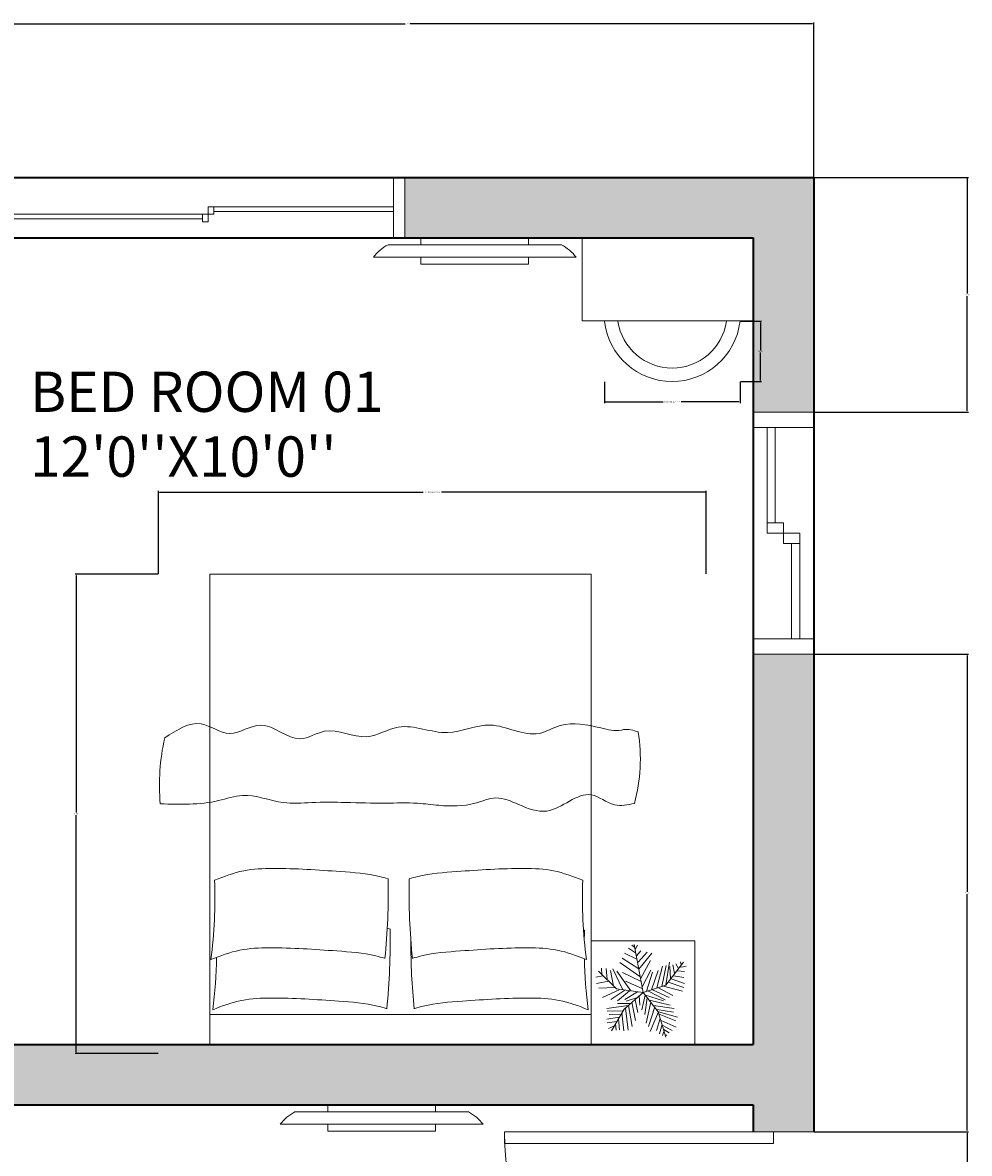
# Model space of a CAD drawing. Units: inches. Extents: x 1789 to 2841, y 3180 to 3702.
# Tile 7 of 14: x 2208 to 2348, y 3510 to 3678. Entities that reach past the tile are written whole.
import ezdxf

# ---------------------------------------------------------------- set-up
doc = ezdxf.new("R2010")
doc.units = ezdxf.units.IN
doc.header["$MEASUREMENT"] = 0
for name, color, linetype, lineweight in [('A-ANNO-DIMS', 2, 'Continuous', 18), ('A-AREA-IDEN', 7, 'Continuous', 18), ('A-EQPM', 8, 'Continuous', 18), ('A-WALL', 40, 'Continuous', 35), ('A-WALL-PATT', 252, 'Continuous', 13), ('DORS', 70, 'Continuous', 18), ('FURNITURE', 34, 'Continuous', 18), ('WINDOWS', 130, 'Continuous', 18)]:
    doc.layers.add(name, color=color, linetype=linetype, lineweight=lineweight)
doc.styles.get("Standard").update_dxf_attribs({"font": 'arial.ttf'})
doc.dimstyles.get("Standard").update_dxf_attribs({"dimtxt": 0.18, "dimasz": 0.18, "dimexe": 0.18, "dimexo": 0.0625, "dimgap": 0.09, "dimtad": 0, "dimtih": 1, "dimtoh": 1, "dimdec": 0, "dimzin": 0, "dimdsep": 46, "dimlunit": 3, "dimtxsty": 'Standard', "dimcen": 0.09, "dimadec": 0, "dimazin": 0, "dimtfac": 1, "dimtdec": 0, "dimtofl": 0, "dimtmove": 0, "dimatfit": 3, "dimfxl": 1, "dimtolj": 1, "dimtzin": 0, "dimarcsym": 0})

# ---------------------------------------------------------------- blocks, each defined once
blk = doc.blocks.new('HYJ')
for p, q in [((2236.02, 3650.77), (2262.74, 3650.77)), ((2206.12, 3649.67), (2234.3, 3649.67)), ((2206.12, 3649), (2234.3, 3649)), ((2236.02, 3650.11), (2262.74, 3650.11))]:
    blk.add_line(p, q)
for points in [[(2204.43, 3646.16), (2264.43, 3646.16), (2264.43, 3655.16), (2204.43, 3655.16)], [(2204.43, 3655.16), (2206.12, 3655.16), (2206.12, 3646.16), (2204.43, 3646.16)], [(2264.43, 3655.16), (2262.74, 3655.16), (2262.74, 3646.16), (2264.43, 3646.16)], [(2235.16, 3650.77), (2236.02, 3650.77), (2236.02, 3649.67), (2235.16, 3649.67)], [(2234.3, 3649.67), (2235.16, 3649.67), (2235.16, 3648.56), (2234.3, 3648.56)]]:
    blk.add_lwpolyline(points, close=True)
blk = doc.blocks.new('KIK')
for p, q in [((2336.3, 3607.04), (2336.3, 3621.23)), ((2337.52, 3607.04), (2337.52, 3621.23)), ((2339.95, 3603.98), (2339.95, 3589.79)), ((2341.17, 3603.98), (2341.17, 3589.79))]:
    blk.add_line(p, q)
for points in [[(2343.23, 3623.51), (2343.23, 3587.51), (2334.23, 3587.51), (2334.23, 3623.51)], [(2343.23, 3623.51), (2334.23, 3623.51), (2334.23, 3621.23), (2343.23, 3621.23)], [(2338.73, 3605.51), (2336.3, 3605.51), (2336.3, 3607.04), (2338.73, 3607.04)], [(2341.17, 3603.98), (2338.73, 3603.98), (2338.73, 3605.51), (2341.17, 3605.51)], [(2343.23, 3587.51), (2334.23, 3587.51), (2334.23, 3589.79), (2343.23, 3589.79)]]:
    blk.add_lwpolyline(points, close=True)
blk = doc.blocks.new('GTGTG')
for points in [[(2266.82, 3646.16), (2282.82, 3646.16), (2282.82, 3645.14), (2266.82, 3645.14)], [(2266.82, 3643.29), (2282.82, 3643.29), (2282.82, 3642.27), (2266.82, 3642.27)]]:
    blk.add_lwpolyline(points, close=True)
for points in [[(2261.92, 3645.14), (2287.72, 3645.14)], [(2289.9, 3643.29), (2259.74, 3643.29)]]:
    blk.add_lwpolyline(points)
for centre, start, end in [((2265.21, 3639.05), 118.4184, 142.2436), ((2284.43, 3639.05), 37.7564, 61.5816)]:
    blk.add_arc(centre, 6.92, start, end)
blk = doc.blocks.new('*U26')
for p, q in [((0, 0), (0, -6)), ((40, 0), (40, -6))]:
    blk.add_line(p, q)
blk.add_lwpolyline([(0, 0), (0, 40), (1.75, 40), (1.75, 0)], close=True)
blk.add_arc((0, 0), 40, 0, 90)
blk = doc.blocks.new('*U22')
for p, q in [((-10.186, 53.64), (-13.084, 55.962)), ((0, 0), (-10.5, 57)), ((-9.099, 51.782), (-6.563, 55.962)), ((-5.114, 28.097), (-24.676, 40.636)), ((-7.288, 39.707), (-21.778, 46.673)), ((-8.737, 47.138), (-17.069, 52.711)), ((-7.65, 43.423), (-2.578, 49.46)), ((-5.839, 35.992), (4.667, 48.067)), ((-5.114, 27.632), (10.463, 46.673)), ((-48.585, 21.131), (-49.309, 29.026)), ((-43.513, 28.561), (-42.427, 15.558)), ((-35.544, 28.097), (-24.314, 3.947)), ((-3.665, 19.273), (-27.574, 35.527)), ((-2.941, 16.486), (8.652, 37.85)), ((16.259, 5.805), (23.142, 31.348)), ((22.055, 7.198), (27.489, 32.277)), ((27, 9), (48, 36)), ((27.127, 9.056), (31.112, 35.992)), ((31.836, 30.883), (32.561, 16.486)), ((35.096, 32.741), (37.27, 22.524)), ((38.719, 34.134), (41.979, 28.561)), ((43.791, 29.954), (51.036, 30.883)), ((44.153, 36.456), (45.239, 32.741)), ((-47.498, 19.737), (-55.83, 18.344)), ((-40.615, 13.7), (-55.105, 10.913)), ((-31.5, 4.5), (-52.5, 25.5)), ((-38.442, 26.239), (-34.819, 7.663)), ((-14.533, 2.09), (-30.834, 25.31)), ((-24.314, 23.917), (-2.941, 13.7)), ((-20.691, 13.7), (-1.129, 4.876)), ((-1.129, 6.734), (9.014, 26.704)), ((3.942, 1.625), (11.187, 24.381)), ((10.101, 3.483), (17.708, 26.239)), ((33.285, 16.486), (48.862, 10.913)), ((36.183, 19.737), (48.137, 17.88)), ((40.53, 25.775), (48.862, 24.846)), ((-33.37, 6.269), (-52.207, 5.34)), ((-28.299, 3.483), (-47.86, -5.805)), ((-21.416, 3.018), (-38.079, -8.128)), ((0, 0), (-31.5, 4.5)), ((-15.982, 2.09), (-30.11, -9.521)), ((0, 0), (-22.5, -19.5)), ((-6.563, 1.161), (-21.416, -8.128)), ((0, 0), (27, 9)), ((0, 0), (18, -22.5)), ((6.478, 1.625), (26.04, -8.592)), ((11.187, 3.483), (30.749, -5.805)), ((18.07, 5.805), (35.096, -3.483)), ((24.229, 7.663), (46.688, 1.625)), ((29.662, 12.307), (48.137, 6.269)), ((-15.257, -12.772), (-30.11, -12.772)), ((-6.563, -5.805), (-19.967, -9.985)), ((-13.446, -11.378), (-8.737, -32.741)), ((-9.461, -8.592), (-6.201, -23.453)), ((-4.752, -3.483), (-3.665, -14.629)), ((2.493, -3.019), (-1.491, -20.202)), ((1.769, -2.555), (24.229, -9.521)), ((5.029, -6.27), (2.131, -25.775)), ((9.014, -11.378), (3.58, -35.992)), ((7.565, -9.056), (32.198, -14.629)), ((-17.431, -15.094), (-42.789, -18.809)), ((-24.314, -21.596), (-42.427, -22.06)), ((-26.849, -26.24), (-40.253, -25.775)), ((-22.5, -19.5), (-37.5, -45)), ((-25.038, -23.918), (-22.865, -45.281)), ((-20.691, -18.345), (-17.793, -44.352)), ((-17.069, -15.094), (-12.721, -40.172)), ((14.085, -16.951), (6.478, -40.172)), ((18.07, -22.524), (8.289, -45.745)), ((12.274, -15.094), (36.907, -18.809)), ((16.259, -19.738), (36.183, -22.989)), ((18, -22.5), (27, -52.5)), ((18.433, -22.524), (40.53, -29.026)), ((19.157, -25.311), (38.719, -33.206)), ((-28.299, -29.026), (-42.789, -31.348)), ((-30.834, -34.135), (-42.427, -35.528)), ((-34.457, -39.708), (-40.978, -42.494)), ((-32.646, -36.921), (-31.921, -44.352)), ((-29.023, -30.884), (-27.936, -43.887)), ((20.244, -30.419), (15.897, -44.816)), ((22.78, -37.85), (19.519, -48.532)), ((21.331, -32.741), (39.081, -40.636)), ((22.78, -38.314), (34.372, -44.816)), ((24.591, -45.745), (23.142, -50.854)), ((24.591, -43.423), (30.749, -47.603)), ((26.764, -49.925), (28.213, -50.854))]:
    blk.add_line(p, q)
blk = doc.blocks.new('BEDD')
for points in [[(2235.4, 3526.16), (2292.14, 3526.16), (2292.14, 3596.12), (2235.4, 3596.12)], [(2292.14, 3526.16), (2307.57, 3526.16), (2307.57, 3541.59), (2292.14, 3541.59)], [(2235.4, 3526.16), (2292.14, 3526.16), (2292.14, 3530.61), (2235.4, 3530.61)]]:
    blk.add_lwpolyline(points, close=True)
for centre, radius, start, end in [((2259.99, 3564.78), 32.07, 167.4063, 185.0216), ((2273.81, 3568.71), 25.64, 344.9042, 8.8372), ((2163.47, 3548.06), 72.69, 352.674, 2.0029), ((2165.57, 3548.81), 96.38, 354.1175, 1.1854), ((2361.42, 3548.81), 96.38, 178.8146, 185.8825), ((2363.52, 3548.06), 72.69, 177.9971, 187.326), ((2165.85, 3541.35), 96.38, 354.1175, 1.1854), ((2363.79, 3540.6), 72.69, 177.9971, 179.1531), ((2361.69, 3541.35), 96.38, 179.877, 185.8825), ((2163.75, 3540.6), 72.69, 352.674, 358.8312), ((2363.79, 3540.6), 72.69, 181.3344, 187.326)]:
    blk.add_arc(centre, radius, start, end)
for points, knots in [([(2228.7, 3571.77), (2230.5, 3572.97), (2233.69, 3575.11), (2238.44, 3571.24), (2243.48, 3575.3), (2248.08, 3570.3), (2253.24, 3573.93), (2258.37, 3570.76), (2264.15, 3574.63), (2270.52, 3571.37), (2277.36, 3575.01), (2283.2, 3571.25), (2288.29, 3574.45), (2292.59, 3573.51), (2295.73, 3572.7), (2297.56, 3573.17), (2298.4, 3572.89), (2299.15, 3572.65)], [0, 0, 0, 0, 5.813057, 10.291797, 15.071674, 21.264477, 25.062958, 31.395117, 36.284741, 43.6566, 50.0956, 57.47363, 60.824937, 66.871309, 69.965772, 70.260383, 72.512122, 72.512122, 72.512122, 72.512122]), ([(2228.05, 3561.97), (2230.96, 3561.87), (2235.09, 3561.73), (2241.08, 3563.86), (2245.67, 3561.8), (2250.85, 3562.25), (2255.91, 3562.17), (2261.15, 3562), (2265.78, 3562.19), (2270.21, 3561.59), (2274.18, 3561.57), (2278.08, 3563.31), (2281.58, 3561.74), (2286.46, 3559.73), (2291.21, 3564.99), (2295.28, 3561.31), (2297.57, 3561.81), (2298.57, 3562.03)], [0, 0, 0, 0, 8.669632, 12.310458, 18.461416, 22.693385, 27.790985, 33.658819, 38.43562, 41.630677, 47.052462, 50.224855, 53.725722, 58.058029, 65.069701, 68.862462, 71.815525, 71.815525, 71.815525, 71.815525]), ([(2236.12, 3550.6), (2237.54, 3551.15), (2240.34, 3552.23), (2246.72, 3552.46), (2253.43, 3551.99), (2259.2, 3551.57), (2261.51, 3550.92), (2261.93, 3550.8)], [0, 0, 0, 0, 4.544245, 8.926813, 18.957656, 24.819591, 26.148375, 26.148375, 26.148375, 26.148375]), ([(2290.87, 3550.6), (2289.45, 3551.15), (2286.65, 3552.23), (2280.27, 3552.46), (2273.56, 3551.99), (2267.8, 3551.57), (2265.49, 3550.92), (2265.06, 3550.8)], [0, 0, 0, 0, 4.544245, 8.926813, 18.957656, 24.819591, 26.148375, 26.148375, 26.148375, 26.148375]), ([(2235.57, 3538.79), (2236.99, 3539.34), (2239.79, 3540.42), (2246.18, 3540.65), (2252.88, 3540.18), (2258.65, 3539.76), (2260.96, 3539.11), (2261.38, 3538.99)], [0, 0, 0, 0, 4.544245, 8.926813, 18.957656, 24.819591, 26.148375, 26.148375, 26.148375, 26.148375]), ([(2291.42, 3538.79), (2290, 3539.34), (2287.2, 3540.42), (2280.82, 3540.65), (2274.11, 3540.18), (2268.34, 3539.76), (2266.03, 3539.11), (2265.61, 3538.99)], [0, 0, 0, 0, 4.544245, 8.926813, 18.957656, 24.819591, 26.148375, 26.148375, 26.148375, 26.148375]), ([(2235.84, 3531.33), (2237.27, 3531.88), (2240.06, 3532.96), (2246.45, 3533.19), (2253.15, 3532.71), (2258.92, 3532.3), (2261.23, 3531.65), (2261.66, 3531.53)], [0, 0, 0, 0, 4.544245, 8.926813, 18.957656, 24.819591, 26.148375, 26.148375, 26.148375, 26.148375]), ([(2291.69, 3531.33), (2290.27, 3531.88), (2287.47, 3532.96), (2281.09, 3533.19), (2274.39, 3532.71), (2268.62, 3532.3), (2266.31, 3531.65), (2265.88, 3531.53)], [0, 0, 0, 0, 4.544245, 8.926813, 18.957656, 24.819591, 26.148375, 26.148375, 26.148375, 26.148375])]:
    blk.add_open_spline(points, degree=3, knots=knots)
for points in [[(2261.81, 3543.46), (2261.94, 3543.42), (2262.07, 3543.38), (2262.21, 3543.34)], [(2291.15, 3543.14), (2291.09, 3543.16), (2291.04, 3543.18), (2290.99, 3543.2)]]:
    blk.add_open_spline(points, degree=3)
at = {"xscale": 0.1258179792922857, "yscale": 0.1258179792922857, "zscale": 0.1258179792922857}
blk.add_blockref('*U22', (2299.85, 3533.87), dxfattribs=at)
blk = doc.blocks.new('CHAIR-DESK-ROUND')
for radius, start, end in [(10.16, 186.7458, 353.2542), (8.16, 188.4094, 351.5906)]:
    blk.add_arc((10.09, 10.16), radius, start, end)
blk = doc.blocks.new('*D55')
at = {"layer": 'A-ANNO-DIMS', "color": 0, "lineweight": -2, "transparency": 16777216}
for p, q in [((2227.76, 3596.18), (2227.76, 3608.52)), ((2227.94, 3608.34), (2267.14, 3608.34)), ((2309.08, 3608.34), (2269.88, 3608.34)), ((2309.26, 3596.18), (2309.26, 3608.52))]:
    blk.add_line(p, q, dxfattribs=at)
at = {"layer": 'A-ANNO-DIMS', "color": 0, "transparency": 16777216}
for points in [[(2227.94, 3608.37), (2227.94, 3608.31), (2227.76, 3608.34)], [(2309.08, 3608.37), (2309.08, 3608.31), (2309.26, 3608.34)]]:
    blk.add_solid(points, dxfattribs=at)
at = {"layer": 'Defpoints', "color": 0, "transparency": 16777216}
for p in [(2309.26, 3608.34), (2227.76, 3596.12), (2309.26, 3596.12)]:
    blk.add_point(p, dxfattribs=at)
at = {"layer": 'A-ANNO-DIMS', "color": 0, "transparency": 16777216, "insert": (2268.51, 3608.34), "char_height": 0.18, "attachment_point": 5}
blk.add_mtext('\\A1;DOUBLE BED 81 TYP.', dxfattribs=at)
blk = doc.blocks.new('*D56')
at = {"layer": 'A-ANNO-DIMS', "color": 0, "lineweight": -2, "transparency": 16777216}
for p, q in [((2227.7, 3596.12), (2215.36, 3596.12)), ((2215.54, 3595.94), (2215.54, 3560.65)), ((2215.54, 3525.01), (2215.54, 3560.29)), ((2227.7, 3524.83), (2215.36, 3524.83))]:
    blk.add_line(p, q, dxfattribs=at)
at = {"layer": 'A-ANNO-DIMS', "color": 0, "transparency": 16777216}
for points in [[(2215.51, 3595.94), (2215.57, 3595.94), (2215.54, 3596.12)], [(2215.51, 3525.01), (2215.57, 3525.01), (2215.54, 3524.83)]]:
    blk.add_solid(points, dxfattribs=at)
at = {"layer": 'Defpoints', "color": 0, "transparency": 16777216}
for p in [(2215.54, 3596.12), (2227.76, 3596.12), (2227.76, 3524.83)]:
    blk.add_point(p, dxfattribs=at)
at = {"layer": 'A-ANNO-DIMS', "color": 0, "transparency": 16777216, "insert": (2215.54, 3560.47), "char_height": 0.18, "attachment_point": 5}
blk.add_mtext('\\A1;71 TYP.', dxfattribs=at)
blk = doc.blocks.new('*D75')
at = {"layer": 'A-ANNO-DIMS', "color": 0, "lineweight": -2, "transparency": 16777216}
for p, q in [((2294.1, 3624.73), (2294.1, 3621.58)), ((2314.28, 3624.73), (2314.28, 3621.58)), ((2294.28, 3621.76), (2302.86, 3621.76)), ((2314.1, 3621.76), (2305.52, 3621.76))]:
    blk.add_line(p, q, dxfattribs=at)
at = {"layer": 'A-ANNO-DIMS', "color": 0, "transparency": 16777216}
for points in [[(2294.28, 3621.79), (2294.28, 3621.73), (2294.1, 3621.76)], [(2314.1, 3621.79), (2314.1, 3621.73), (2314.28, 3621.76)]]:
    blk.add_solid(points, dxfattribs=at)
at = {"layer": 'Defpoints', "color": 0, "transparency": 16777216}
for p in [(2294.1, 3624.79), (2314.28, 3624.79), (2314.28, 3621.76)]:
    blk.add_point(p, dxfattribs=at)
at = {"layer": 'A-ANNO-DIMS', "color": 0, "transparency": 16777216, "insert": (2304.19, 3621.76), "char_height": 0.18, "attachment_point": 5}
blk.add_mtext('\\A1;DESK CHAIR 20 TYP.', dxfattribs=at)
blk = doc.blocks.new('*D76')
at = {"layer": 'A-ANNO-DIMS', "color": 0, "lineweight": -2, "transparency": 16777216}
for p, q in [((2314.34, 3633.76), (2317.49, 3633.76)), ((2317.31, 3633.58), (2317.31, 3629.46)), ((2317.31, 3624.97), (2317.31, 3629.09)), ((2314.34, 3624.79), (2317.49, 3624.79))]:
    blk.add_line(p, q, dxfattribs=at)
at = {"layer": 'A-ANNO-DIMS', "color": 0, "transparency": 16777216}
for points in [[(2317.28, 3633.58), (2317.34, 3633.58), (2317.31, 3633.76)], [(2317.28, 3624.97), (2317.34, 3624.97), (2317.31, 3624.79)]]:
    blk.add_solid(points, dxfattribs=at)
at = {"layer": 'Defpoints', "color": 0, "transparency": 16777216}
for p in [(2314.28, 3633.76), (2317.31, 3633.76), (2314.28, 3624.79)]:
    blk.add_point(p, dxfattribs=at)
at = {"layer": 'A-ANNO-DIMS', "color": 0, "transparency": 16777216, "insert": (2317.31, 3629.28), "char_height": 0.18, "attachment_point": 5}
blk.add_mtext('\\A1;9 TYP.', dxfattribs=at)
blk = doc.blocks.new('*D85')
at = {"layer": 'A-ANNO-DIMS', "color": 0, "lineweight": -2, "transparency": 16777216}
for p, q in [((2204.43, 3655.22), (2204.43, 3678.19)), ((2204.61, 3678.01), (2264.45, 3678.01)), ((2325.05, 3678.01), (2265.22, 3678.01)), ((2325.23, 3655.22), (2325.23, 3678.19))]:
    blk.add_line(p, q, dxfattribs=at)
at = {"layer": 'A-ANNO-DIMS', "color": 0, "transparency": 16777216}
for points in [[(2204.61, 3678.04), (2204.61, 3677.98), (2204.43, 3678.01)], [(2325.05, 3678.04), (2325.05, 3677.98), (2325.23, 3678.01)]]:
    blk.add_solid(points, dxfattribs=at)
at = {"layer": 'Defpoints', "color": 0, "transparency": 16777216}
for p in [(2325.23, 3678.01), (2204.43, 3655.16), (2325.23, 3655.16)]:
    blk.add_point(p, dxfattribs=at)
at = {"layer": 'A-ANNO-DIMS', "color": 0, "transparency": 16777216, "insert": (2264.83, 3678.01), "char_height": 0.18, "attachment_point": 5}
blk.add_mtext('\\A1;120.8', dxfattribs=at)
blk = doc.blocks.new('*D86')
at = {"layer": 'A-ANNO-DIMS', "color": 0, "lineweight": -2, "transparency": 16777216}
for p, q in [((2325.3, 3655.16), (2348.26, 3655.16)), ((2348.08, 3654.98), (2348.08, 3637.88)), ((2348.08, 3620.41), (2348.08, 3637.51)), ((2325.3, 3620.23), (2348.26, 3620.23))]:
    blk.add_line(p, q, dxfattribs=at)
at = {"layer": 'A-ANNO-DIMS', "color": 0, "transparency": 16777216}
for points in [[(2348.05, 3654.98), (2348.11, 3654.98), (2348.08, 3655.16)], [(2348.05, 3620.41), (2348.11, 3620.41), (2348.08, 3620.23)]]:
    blk.add_solid(points, dxfattribs=at)
at = {"layer": 'Defpoints', "color": 0, "transparency": 16777216}
for p in [(2325.23, 3655.16), (2325.23, 3620.23), (2348.08, 3620.23)]:
    blk.add_point(p, dxfattribs=at)
at = {"layer": 'A-ANNO-DIMS', "color": 0, "transparency": 16777216, "insert": (2348.08, 3637.69), "char_height": 0.18, "attachment_point": 5}
blk.add_mtext('\\A1;34.93', dxfattribs=at)
blk = doc.blocks.new('*D87')
at = {"layer": 'A-ANNO-DIMS', "color": 0, "lineweight": -2, "transparency": 16777216}
for p, q in [((2325.3, 3584.23), (2348.26, 3584.23)), ((2348.08, 3584.05), (2348.08, 3548.88)), ((2348.08, 3513.34), (2348.08, 3548.51)), ((2325.3, 3513.16), (2348.26, 3513.16))]:
    blk.add_line(p, q, dxfattribs=at)
at = {"layer": 'A-ANNO-DIMS', "color": 0, "transparency": 16777216}
for points in [[(2348.05, 3584.05), (2348.11, 3584.05), (2348.08, 3584.23)], [(2348.05, 3513.34), (2348.11, 3513.34), (2348.08, 3513.16)]]:
    blk.add_solid(points, dxfattribs=at)
at = {"layer": 'Defpoints', "color": 0, "transparency": 16777216}
for p in [(2325.23, 3584.23), (2325.23, 3513.16), (2348.08, 3513.16)]:
    blk.add_point(p, dxfattribs=at)
at = {"layer": 'A-ANNO-DIMS', "color": 0, "transparency": 16777216, "insert": (2348.08, 3548.69), "char_height": 0.18, "attachment_point": 5}
blk.add_mtext('\\A1;71.07', dxfattribs=at)
blk = doc.blocks.new('*D88')
at = {"layer": 'A-ANNO-DIMS', "color": 0, "lineweight": -2, "transparency": 16777216}
for p, q in [((2325.3, 3513.16), (2348.26, 3513.16)), ((2348.08, 3512.98), (2348.08, 3493.34)), ((2348.08, 3473.34), (2348.08, 3492.98)), ((2325.3, 3473.16), (2348.26, 3473.16))]:
    blk.add_line(p, q, dxfattribs=at)
at = {"layer": 'A-ANNO-DIMS', "color": 0, "transparency": 16777216}
for points in [[(2348.05, 3512.98), (2348.11, 3512.98), (2348.08, 3513.16)], [(2348.05, 3473.34), (2348.11, 3473.34), (2348.08, 3473.16)]]:
    blk.add_solid(points, dxfattribs=at)
at = {"layer": 'Defpoints', "color": 0, "transparency": 16777216}
for p in [(2325.23, 3513.16), (2325.23, 3473.16), (2348.08, 3473.16)]:
    blk.add_point(p, dxfattribs=at)
at = {"layer": 'A-ANNO-DIMS', "color": 0, "transparency": 16777216, "insert": (2348.08, 3493.16), "char_height": 0.18, "attachment_point": 5}
blk.add_mtext('\\A1;40', dxfattribs=at)

msp = doc.modelspace()

# ---------------------------------------------------------------- hatches: boundary and pattern name
at = {"layer": 'A-WALL-PATT'}
h = msp.add_hatch(color=256, dxfattribs=at)
h.dxf.hatch_style = 1
h.paths.add_polyline_path([(2052.2333, 3646.1608), (2052.2333, 3655.1608), (1959.2333, 3655.1608), (1959.2333, 3622.3936), (1968.2333, 3622.3936), (1968.2333, 3646.1608)])
h.paths.add_polyline_path([(2163.2333, 3646.1608), (2163.2333, 3640.1475), (2163.2333, 3568.1608), (2159.2333, 3568.1608), (2159.2333, 3565.4274), (2163.2333, 3565.4274), (2163.2333, 3564.1608), (2169.2333, 3564.1608, -0.02086055), (2172.2333, 3564.0356), (2172.2333, 3646.1608), (2196.2333, 3646.1608), (2204.4325, 3646.1608), (2204.4325, 3655.1608), (2117.6786, 3655.1608), (2117.6786, 3646.1608)])
h.paths.add_polyline_path([(2085.2333, 3646.1608), (2093.6786, 3646.1608), (2093.6786, 3655.1608), (2076.2333, 3655.1608), (2076.2333, 3646.1608), (2076.2333, 3621.0865), (2076.2333, 3526.1608), (2074.2333, 3526.1608), (2074.2333, 3523.1608), (2074.2333, 3517.1608), (2085.2333, 3517.1608), (2085.2333, 3565.4274), (2129.2333, 3565.4274), (2129.2333, 3568.1608), (2085.2333, 3568.1608)])
h.paths.add_polyline_path([(2172.2333, 3526.1608), (2172.2333, 3528.1608), (2163.2333, 3528.1608), (2163.2333, 3517.1608), (2316.2333, 3517.1608), (2316.2333, 3513.1608), (2319.2333, 3513.1608), (2325.2333, 3513.1608), (2325.2333, 3584.2279), (2316.2333, 3584.2279), (2316.2333, 3526.1608)])
h.paths.add_polyline_path([(2325.2333, 3655.1608), (2264.4325, 3655.1608), (2264.4325, 3646.1608), (2316.2333, 3646.1608), (2316.2333, 3633.8369), (2316.2333, 3620.2279), (2325.2333, 3620.2279)])

# ---------------------------------------------------------------- linework, layer by layer
at = {"layer": 'A-WALL'}
for p, q in [((1959.2333, 3655.1608), (2325.2333, 3655.1608)), ((2325.2333, 3655.1608), (2325.2333, 3513.1608)), ((2172.2333, 3646.1608), (2316.2333, 3646.1608)), ((2316.2333, 3646.1608), (2316.2333, 3526.1608)), ((2172.2333, 3526.1608), (2316.2333, 3526.1608)), ((2163.2333, 3517.1608), (2316.2333, 3517.1608)), ((2316.2333, 3517.1608), (2316.2333, 3513.1608))]:
    msp.add_line(p, q, dxfattribs=at)
at = {"layer": 'FURNITURE'}
msp.add_lwpolyline([(2316.2333, 3646.1608), (2290.7859, 3646.1608), (2290.7859, 3633.8369), (2316.2333, 3633.8369)], close=True, dxfattribs=at)

# ---------------------------------------------------------------- block references
at = {"layer": 'A-EQPM'}
for p in [(0, 0), (-13.8545, -129)]:
    msp.add_blockref('GTGTG', p, dxfattribs=at)
at = {"layer": 'DORS', "xscale": -1, "rotation": 90}
msp.add_blockref('*U26', (2319.2333, 3513.1608), dxfattribs=at)
at = {"layer": 'FURNITURE'}
for name, p in [('CHAIR-DESK-ROUND', (2294.097, 3624.79)), ('BEDD', (0, 0))]:
    msp.add_blockref(name, p, dxfattribs=at)
at = {"layer": 'WINDOWS'}
for name, p in [('HYJ', (0, 0)), ('KIK', (-18, -3.2831))]:
    msp.add_blockref(name, p, dxfattribs=at)

# ---------------------------------------------------------------- texts
at = {"layer": 'A-ANNO-DIMS'}
msp.add_text("12'0''X10'0''", height=6, dxfattribs=at).set_placement((2208.6596, 3610.628))
at = {"layer": 'A-AREA-IDEN'}
msp.add_text('BED ROOM 01', height=6, dxfattribs=at).set_placement((2208.6596, 3620.2665))

# ---------------------------------------------------------------- dimensions: what is measured, and where the dimension line sits
at = {"layer": 'A-ANNO-DIMS'}
dim = msp.add_linear_dim(base=(2325.2333, 3678.0108), p1=(2204.4325, 3655.1608), p2=(2325.2333, 3655.1608), dimstyle='Standard', override={"dimdec": 1, "dimlfac": 1, "dimrnd": 0, "dimzin": 0, "dimdsep": 46, "dimlunit": 2}, dxfattribs=at)
dim.commit()
dim.dimension.update_dxf_attribs({"geometry": '*D85', "text_midpoint": (2264.8329, 3678.0108)})
for base, p1, p2, override, picture, middle in [((2348.0833, 3620.2279), (2325.2333, 3655.1608), (2325.2333, 3620.2279), {"dimdec": 2, "dimlfac": 1, "dimrnd": 0, "dimzin": 0, "dimdsep": 46, "dimlunit": 2}, '*D86', (2348.0833, 3637.6943)), ((2348.0833, 3513.1608), (2325.2333, 3584.2279), (2325.2333, 3513.1608), {"dimdec": 2, "dimlfac": 1, "dimrnd": 0, "dimzin": 0, "dimdsep": 46, "dimlunit": 2}, '*D87', (2348.0833, 3548.6943)), ((2348.0833, 3473.1608), (2325.2333, 3513.1608), (2325.2333, 3473.1608), {"dimdec": 0, "dimlfac": 1, "dimrnd": 0, "dimzin": 0, "dimdsep": 46, "dimlunit": 2}, '*D88', (2348.0833, 3493.1608))]:
    dim = msp.add_linear_dim(base=base, p1=p1, p2=p2, angle=90, dimstyle='Standard', override=override, dxfattribs=at)
    dim.commit()
    dim.dimension.update_dxf_attribs({"geometry": picture, "text_midpoint": middle})
for base, p1, p2, picture, middle in [((2317.3092, 3633.7595), (2314.2815, 3624.7905), (2314.2815, 3633.7595), '*D76', (2317.3092, 3629.275)), ((2215.5388, 3596.1187), (2227.763, 3524.83), (2227.763, 3596.1187), '*D56', (2215.5388, 3560.4744))]:
    dim = msp.add_linear_dim(base=base, p1=p1, p2=p2, angle=90, text='<> TYP.', dimstyle='Standard', override={"dimdec": 0, "dimlfac": 1, "dimrnd": 0, "dimzin": 0, "dimdsep": 46, "dimlunit": 2}, dxfattribs=at)
    dim.commit()
    dim.dimension.update_dxf_attribs({"geometry": picture, "text_midpoint": middle})
for base, p1, p2, text, picture, middle in [((2314.2815, 3621.7628), (2294.0966, 3624.7905), (2314.2815, 3624.7905), 'DESK CHAIR <> TYP.', '*D75', (2304.1891, 3621.7628)), ((2309.2583, 3608.343), (2227.763, 3596.1187), (2309.2583, 3596.1187), 'DOUBLE BED <> TYP.', '*D55', (2268.5107, 3608.343))]:
    dim = msp.add_linear_dim(base=base, p1=p1, p2=p2, text=text, dimstyle='Standard', override={"dimdec": 0, "dimlfac": 1, "dimrnd": 0, "dimzin": 0, "dimdsep": 46, "dimlunit": 2}, dxfattribs=at)
    dim.commit()
    dim.dimension.update_dxf_attribs({"geometry": picture, "text_midpoint": middle})

doc.saveas('drawing.dxf')
